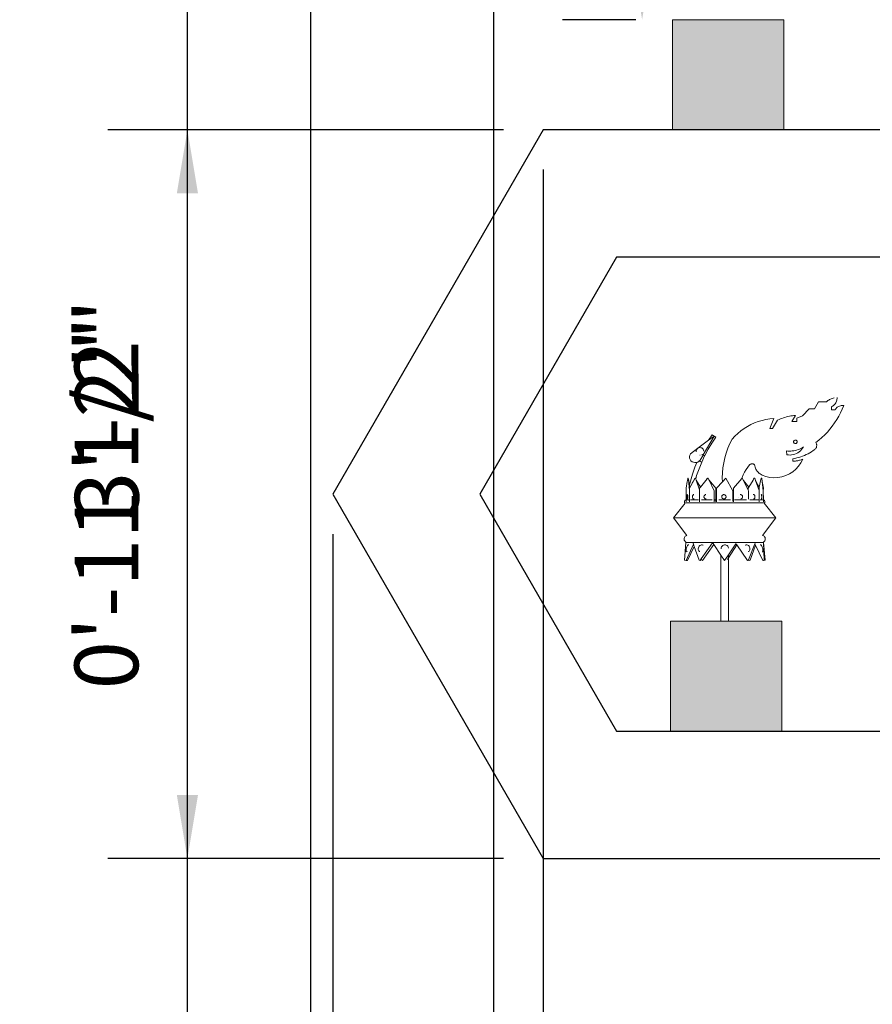
# Model space of a CAD drawing. Units: millimetres. Extents: x 7894 to 8038, y 6851 to 6951.
# Tile 23 of 49: x 7935.52 to 7948.9, y 6916.43 to 6931.89. Entities that reach past the tile are written whole.
import ezdxf

# ---------------------------------------------------------------- set-up
doc = ezdxf.new("R2010")
doc.units = ezdxf.units.MM
for name, color, linetype, lineweight in [('A-ANNO-DIMS', 2, 'Continuous', 18), ('A-FURN-ACCS', 8, 'Continuous', 13), ('A-FURN-CASE', 7, 'Continuous', 30)]:
    doc.layers.add(name, color=color, linetype=linetype, lineweight=lineweight)
doc.layers.add('A-FURN-ACCS-PATT', color=116, linetype='Continuous', lineweight=9, true_color=0x136734)
doc.styles.get("Standard").update_dxf_attribs({"font": 'arial.ttf'})
doc.dimstyles.new('ISO-25', dxfattribs={"dimtxt": 1, "dimasz": 1, "dimexe": 1.25, "dimexo": 0.625, "dimtad": 1, "dimdec": 0, "dimlunit": 4, "dimtxsty": 'Standard', "dimcen": 2.5, "dimclrt": 1, "dimadec": 0, "dimazin": 0, "dimtfac": 1, "dimtdec": 0, "dimtmove": 0, "dimatfit": 3, "dimfxl": 1, "dimarcsym": 0})

# ---------------------------------------------------------------- blocks, each defined once
blk = doc.blocks.new('DISPLAY-LEAF-FINIAL')
for p, q in [((2.209, 3.334), (2.276, 3.441)), ((2.276, 3.441), (2.398, 3.441)), ((2.398, 3.441), (2.409, 3.452)), ((2.409, 3.452), (2.421, 3.461)), ((2.421, 3.461), (2.434, 3.47)), ((2.434, 3.47), (2.447, 3.478)), ((2.447, 3.478), (2.461, 3.485)), ((2.461, 3.485), (2.475, 3.491)), ((2.475, 3.491), (2.489, 3.496)), ((2.489, 3.496), (2.504, 3.501)), ((2.504, 3.501), (2.519, 3.504)), ((2.527, 3.4), (2.516, 3.389)), ((2.536, 3.411), (2.527, 3.4)), ((2.544, 3.424), (2.536, 3.411)), ((2.551, 3.437), (2.544, 3.424)), ((2.556, 3.45), (2.551, 3.437)), ((2.56, 3.465), (2.556, 3.45)), ((2.563, 3.479), (2.56, 3.465)), ((2.565, 3.494), (2.563, 3.479)), ((2.565, 3.508), (2.565, 3.494)), ((2.023, 3.221), (2.127, 3.334)), ((2.127, 3.334), (2.209, 3.334)), ((2.493, 3.371), (2.48, 3.364)), ((2.48, 3.364), (2.48, 3.316)), ((2.48, 3.316), (2.533, 3.316)), ((2.505, 3.379), (2.493, 3.371)), ((2.516, 3.389), (2.505, 3.379)), ((2.533, 3.316), (2.54, 3.327)), ((2.54, 3.327), (2.549, 3.338)), ((2.549, 3.338), (2.558, 3.347)), ((2.558, 3.347), (2.569, 3.356)), ((2.569, 3.356), (2.58, 3.363)), ((2.58, 3.363), (2.592, 3.37)), ((2.62, 3.27), (2.591, 3.216)), ((2.592, 3.37), (2.604, 3.375)), ((2.604, 3.375), (2.617, 3.379)), ((2.617, 3.379), (2.63, 3.382)), ((2.646, 3.325), (2.62, 3.27)), ((2.63, 3.382), (2.643, 3.383)), ((2.643, 3.383), (2.657, 3.383)), ((2.67, 3.382), (2.646, 3.325)), ((2.657, 3.383), (2.67, 3.382)), ((1.213, 3.085), (1.27, 3.111)), ((1.27, 3.111), (1.328, 3.133)), ((1.328, 3.133), (1.388, 3.15)), ((1.388, 3.15), (1.449, 3.164)), ((1.449, 3.164), (1.51, 3.173)), ((1.51, 3.173), (1.572, 3.179)), ((1.572, 3.179), (1.511, 3.024)), ((1.55, 3.024), (1.632, 3.152)), ((1.632, 3.152), (1.654, 3.163)), ((1.654, 3.163), (1.676, 3.173)), ((1.676, 3.173), (1.699, 3.182)), ((1.699, 3.182), (1.722, 3.191)), ((1.722, 3.191), (1.745, 3.198)), ((1.745, 3.198), (1.769, 3.205)), ((1.769, 3.205), (1.793, 3.211)), ((1.793, 3.211), (1.817, 3.216)), ((1.817, 3.216), (1.841, 3.22)), ((1.841, 3.22), (1.865, 3.223)), ((1.914, 3.227), (1.854, 3.133)), ((1.854, 3.133), (1.934, 3.133)), ((1.865, 3.223), (1.889, 3.226)), ((1.889, 3.226), (1.914, 3.227)), ((1.934, 3.185), (2.023, 3.221)), ((1.934, 3.133), (1.934, 3.185)), ((2.527, 3.112), (2.491, 3.062)), ((2.56, 3.163), (2.527, 3.112)), ((2.591, 3.216), (2.56, 3.163)), ((0.962, 2.903), (1.007, 2.946)), ((1.007, 2.946), (1.055, 2.986)), ((1.055, 2.986), (1.105, 3.023)), ((1.105, 3.023), (1.158, 3.056)), ((1.158, 3.056), (1.213, 3.085)), ((1.511, 3.024), (1.55, 3.024)), ((2.413, 2.967), (2.371, 2.923)), ((2.453, 3.014), (2.413, 2.967)), ((2.491, 3.062), (2.453, 3.014)), ((0.547, 2.84), (0.379, 2.713)), ((0.634, 2.9), (0.463, 2.609)), ((0.541, 2.696), (0.599, 2.791)), ((0.605, 2.924), (0.547, 2.84)), ((0.634, 2.905), (0.547, 2.84)), ((0.599, 2.791), (0.663, 2.885)), ((0.634, 2.905), (0.605, 2.924)), ((0.634, 2.9), (0.634, 2.905)), ((0.663, 2.885), (0.634, 2.905)), ((0.884, 2.786), (0.853, 2.713)), ((0.92, 2.857), (0.884, 2.786)), ((0.92, 2.857), (0.962, 2.903)), ((1.883, 2.817), (1.885, 2.824)), ((1.883, 2.81), (1.883, 2.817)), ((1.885, 2.803), (1.883, 2.81)), ((1.885, 2.824), (1.889, 2.831)), ((1.888, 2.797), (1.885, 2.803)), ((1.894, 2.791), (1.888, 2.797)), ((1.889, 2.831), (1.894, 2.836)), ((1.894, 2.836), (1.9, 2.839)), ((1.9, 2.788), (1.894, 2.791)), ((1.9, 2.839), (1.907, 2.841)), ((1.907, 2.786), (1.9, 2.788)), ((1.907, 2.841), (1.914, 2.841)), ((1.914, 2.786), (1.907, 2.786)), ((1.914, 2.841), (1.921, 2.839)), ((1.921, 2.788), (1.914, 2.786)), ((1.921, 2.839), (1.928, 2.836)), ((1.928, 2.791), (1.921, 2.788)), ((1.928, 2.836), (1.933, 2.83)), ((1.933, 2.796), (1.928, 2.791)), ((1.933, 2.83), (1.937, 2.824)), ((1.936, 2.803), (1.933, 2.796)), ((1.938, 2.81), (1.936, 2.803)), ((1.937, 2.824), (1.938, 2.817)), ((1.938, 2.817), (1.938, 2.81)), ((2.281, 2.839), (2.233, 2.801)), ((2.233, 2.801), (2.238, 2.792)), ((2.238, 2.792), (2.242, 2.783)), ((2.242, 2.783), (2.245, 2.774)), ((2.327, 2.88), (2.281, 2.839)), ((2.371, 2.923), (2.327, 2.88)), ((0.264, 2.627), (0.253, 2.607)), ((0.379, 2.713), (0.264, 2.627)), ((0.353, 2.675), (0.358, 2.69)), ((0.353, 2.66), (0.353, 2.675)), ((0.353, 2.659), (0.353, 2.66)), ((0.353, 2.657), (0.353, 2.659)), ((0.358, 2.69), (0.367, 2.703)), ((0.367, 2.703), (0.379, 2.713)), ((0.379, 2.713), (0.393, 2.72)), ((0.393, 2.72), (0.409, 2.723)), ((0.409, 2.723), (0.425, 2.722)), ((0.425, 2.722), (0.44, 2.718)), ((0.44, 2.718), (0.453, 2.709)), ((0.453, 2.709), (0.464, 2.698)), ((0.464, 2.698), (0.471, 2.684)), ((0.471, 2.684), (0.475, 2.669)), ((0.474, 2.667), (0.475, 2.669)), ((0.474, 2.667), (0.475, 2.666)), ((0.541, 2.696), (0.488, 2.597)), ((0.826, 2.638), (0.804, 2.562)), ((0.853, 2.713), (0.826, 2.638)), ((1.793, 2.668), (1.77, 2.67)), ((1.77, 2.67), (1.776, 2.611)), ((1.816, 2.667), (1.793, 2.668)), ((1.84, 2.668), (1.816, 2.667)), ((1.863, 2.67), (1.84, 2.668)), ((1.886, 2.673), (1.863, 2.67)), ((1.909, 2.678), (1.886, 2.673)), ((1.926, 2.63), (1.902, 2.62)), ((1.931, 2.684), (1.909, 2.678)), ((1.949, 2.642), (1.926, 2.63)), ((1.954, 2.692), (1.931, 2.684)), ((1.97, 2.657), (1.949, 2.642)), ((1.975, 2.701), (1.954, 2.692)), ((1.99, 2.673), (1.97, 2.657)), ((1.996, 2.711), (1.975, 2.701)), ((2.007, 2.692), (1.99, 2.673)), ((2.017, 2.722), (1.996, 2.711)), ((2.023, 2.712), (2.007, 2.692)), ((2.036, 2.734), (2.017, 2.722)), ((2.036, 2.734), (2.023, 2.712)), ((2.11, 2.627), (2.082, 2.613)), ((2.137, 2.643), (2.11, 2.627)), ((2.164, 2.659), (2.137, 2.643)), ((2.19, 2.677), (2.164, 2.659)), ((2.216, 2.695), (2.19, 2.677)), ((2.223, 2.702), (2.216, 2.695)), ((2.23, 2.709), (2.223, 2.702)), ((2.235, 2.717), (2.23, 2.709)), ((2.24, 2.726), (2.235, 2.717)), ((2.243, 2.735), (2.24, 2.726)), ((2.245, 2.745), (2.243, 2.735)), ((2.245, 2.774), (2.246, 2.764)), ((2.246, 2.754), (2.245, 2.745)), ((2.246, 2.764), (2.246, 2.754)), ((0.253, 2.607), (0.249, 2.584)), ((0.249, 2.58), (0.249, 2.584)), ((0.249, 2.58), (0.251, 2.557)), ((0.251, 2.557), (0.259, 2.536)), ((0.259, 2.536), (0.272, 2.517)), ((0.272, 2.517), (0.29, 2.502)), ((0.29, 2.502), (0.311, 2.492)), ((0.311, 2.492), (0.334, 2.488)), ((0.363, 2.491), (0.332, 2.415)), ((0.334, 2.488), (0.358, 2.489)), ((0.358, 2.489), (0.363, 2.491)), ((0.363, 2.491), (0.38, 2.497)), ((0.365, 2.496), (0.363, 2.491)), ((0.38, 2.497), (0.4, 2.51)), ((0.398, 2.513), (0.402, 2.512)), ((0.398, 2.391), (0.44, 2.495)), ((0.403, 2.513), (0.4, 2.514)), ((0.4, 2.51), (0.402, 2.512)), ((0.402, 2.512), (0.403, 2.513)), ((0.402, 2.512), (0.44, 2.495)), ((0.403, 2.513), (0.415, 2.527)), ((0.403, 2.513), (0.44, 2.496)), ((0.409, 2.511), (0.408, 2.509)), ((0.42, 2.535), (0.409, 2.511)), ((0.414, 2.606), (0.413, 2.603)), ((0.461, 2.605), (0.415, 2.527)), ((0.44, 2.496), (0.486, 2.593)), ((0.443, 2.613), (0.446, 2.612)), ((0.451, 2.615), (0.449, 2.616)), ((0.463, 2.609), (0.461, 2.605)), ((0.486, 2.593), (0.461, 2.605)), ((0.463, 2.609), (0.488, 2.597)), ((0.787, 2.485), (0.774, 2.406)), ((0.804, 2.562), (0.787, 2.485)), ((1.801, 2.608), (1.776, 2.611)), ((1.827, 2.607), (1.801, 2.608)), ((1.852, 2.609), (1.827, 2.607)), ((1.878, 2.613), (1.852, 2.609)), ((1.903, 2.554), (1.872, 2.548)), ((1.872, 2.548), (1.872, 2.508)), ((1.872, 2.508), (1.885, 2.509)), ((1.902, 2.62), (1.878, 2.613)), ((1.885, 2.509), (1.898, 2.51)), ((1.898, 2.51), (1.911, 2.511)), ((1.934, 2.561), (1.903, 2.554)), ((1.911, 2.511), (1.924, 2.513)), ((1.924, 2.513), (1.937, 2.515)), ((1.964, 2.569), (1.934, 2.561)), ((1.937, 2.515), (1.95, 2.518)), ((1.95, 2.518), (1.963, 2.521)), ((1.997, 2.484), (1.961, 2.432)), ((1.963, 2.521), (1.976, 2.524)), ((1.994, 2.578), (1.964, 2.569)), ((1.976, 2.524), (1.988, 2.528)), ((1.988, 2.528), (2.001, 2.532)), ((2.024, 2.588), (1.994, 2.578)), ((2.026, 2.541), (1.997, 2.484)), ((2.001, 2.532), (2.013, 2.536)), ((2.013, 2.536), (2.026, 2.541)), ((2.053, 2.6), (2.024, 2.588)), ((2.082, 2.613), (2.053, 2.6)), ((0.332, 2.415), (0.295, 2.306)), ((0.361, 2.285), (0.398, 2.391)), ((0.766, 2.327), (0.763, 2.248)), ((0.774, 2.406), (0.766, 2.327)), ((1.113, 2.339), (1.092, 2.297)), ((1.136, 2.379), (1.113, 2.339)), ((1.163, 2.417), (1.136, 2.379)), ((1.193, 2.452), (1.163, 2.417)), ((1.198, 2.457), (1.193, 2.452)), ((1.204, 2.462), (1.198, 2.457)), ((1.211, 2.465), (1.204, 2.462)), ((1.218, 2.467), (1.211, 2.465)), ((1.225, 2.469), (1.218, 2.467)), ((1.232, 2.47), (1.225, 2.469)), ((1.239, 2.469), (1.232, 2.47)), ((1.247, 2.467), (1.239, 2.469)), ((1.254, 2.465), (1.247, 2.467)), ((1.26, 2.462), (1.254, 2.465)), ((1.266, 2.457), (1.26, 2.462)), ((1.271, 2.452), (1.266, 2.457)), ((1.274, 2.435), (1.271, 2.452)), ((1.278, 2.418), (1.274, 2.435)), ((1.283, 2.402), (1.278, 2.418)), ((1.29, 2.386), (1.283, 2.402)), ((1.298, 2.371), (1.29, 2.386)), ((1.308, 2.357), (1.298, 2.371)), ((1.319, 2.343), (1.308, 2.357)), ((1.331, 2.331), (1.319, 2.343)), ((1.343, 2.319), (1.331, 2.331)), ((1.357, 2.309), (1.343, 2.319)), ((1.87, 2.344), (1.816, 2.31)), ((1.918, 2.385), (1.87, 2.344)), ((1.961, 2.432), (1.918, 2.385)), ((0.213, 2.19), (0.195, 2.086)), ((0.213, 2.19), (0.215, 2.201)), ((0.215, 2.201), (0.22, 2.245)), ((0.223, 2.245), (0.215, 2.201)), ((0.223, 2.245), (0.22, 2.245)), ((0.223, 2.245), (0.23, 2.245)), ((0.232, 2.22), (0.23, 2.245)), ((0.232, 2.22), (0.25, 2.138)), ((0.244, 2.11), (0.232, 2.22)), ((0.317, 2.207), (0.248, 2.086)), ((0.263, 2.194), (0.25, 2.138)), ((0.295, 2.306), (0.263, 2.194)), ((0.297, 2.185), (0.292, 2.162)), ((0.317, 2.207), (0.33, 2.245)), ((0.338, 2.245), (0.317, 2.207)), ((0.332, 2.245), (0.33, 2.245)), ((0.344, 2.245), (0.338, 2.245)), ((0.347, 2.235), (0.344, 2.245)), ((0.347, 2.235), (0.361, 2.285)), ((0.354, 2.213), (0.347, 2.235)), ((0.354, 2.213), (0.42, 2.104)), ((0.404, 2.061), (0.354, 2.213)), ((0.507, 2.209), (0.42, 2.104)), ((0.507, 2.209), (0.525, 2.245)), ((0.532, 2.239), (0.507, 2.209)), ((0.528, 2.245), (0.525, 2.245)), ((0.528, 2.245), (0.532, 2.239)), ((0.537, 2.245), (0.532, 2.239)), ((0.54, 2.245), (0.537, 2.245)), ((0.556, 2.211), (0.54, 2.245)), ((0.548, 2.22), (0.556, 2.211)), ((0.556, 2.211), (0.663, 2.086)), ((0.636, 2.045), (0.556, 2.211)), ((0.765, 2.186), (0.671, 2.086)), ((0.763, 2.248), (0.765, 2.186)), ((0.821, 2.245), (0.765, 2.186)), ((0.93, 2.045), (0.821, 2.245)), ((1.07, 2.239), (0.939, 2.086)), ((1.07, 2.239), (1.069, 2.235)), ((1.071, 2.24), (1.07, 2.239)), ((1.07, 2.239), (1.071, 2.237)), ((1.075, 2.254), (1.071, 2.24)), ((1.074, 2.245), (1.071, 2.24)), ((1.074, 2.245), (1.078, 2.245)), ((1.092, 2.297), (1.075, 2.254)), ((1.095, 2.209), (1.078, 2.245)), ((1.095, 2.209), (1.182, 2.104)), ((1.095, 2.209), (1.171, 2.054)), ((1.248, 2.213), (1.182, 2.104)), ((1.248, 2.213), (1.258, 2.245)), ((1.265, 2.242), (1.248, 2.213)), ((1.258, 2.245), (1.264, 2.245)), ((1.264, 2.245), (1.265, 2.242)), ((1.267, 2.245), (1.265, 2.242)), ((1.267, 2.245), (1.272, 2.245)), ((1.285, 2.207), (1.272, 2.245)), ((1.285, 2.207), (1.344, 2.103)), ((1.285, 2.207), (1.34, 2.048)), ((1.37, 2.22), (1.344, 2.103)), ((1.372, 2.3), (1.357, 2.309)), ((1.37, 2.22), (1.372, 2.245)), ((1.375, 2.245), (1.37, 2.22)), ((1.387, 2.292), (1.372, 2.3)), ((1.372, 2.245), (1.375, 2.245)), ((1.375, 2.245), (1.382, 2.245)), ((1.382, 2.245), (1.389, 2.19)), ((1.447, 2.27), (1.387, 2.292)), ((1.389, 2.19), (1.408, 2.086)), ((1.407, 2.045), (1.389, 2.19)), ((1.509, 2.256), (1.447, 2.27)), ((1.572, 2.25), (1.509, 2.256)), ((1.635, 2.253), (1.572, 2.25)), ((1.698, 2.264), (1.635, 2.253)), ((1.759, 2.283), (1.698, 2.264)), ((1.816, 2.31), (1.759, 2.283)), ((0.195, 2.086), (0.195, 2.048)), ((0.195, 2.045), (0.195, 2.048)), ((0.195, 2.045), (0.195, 1.903)), ((0.244, 2.11), (0.239, 2.089)), ((0.25, 2.138), (0.244, 2.11)), ((0.248, 2.065), (0.244, 2.11)), ((0.248, 2.086), (0.248, 2.065)), ((0.248, 2.065), (0.248, 1.903)), ((0.25, 2.138), (0.256, 2.115)), ((0.42, 2.104), (0.404, 2.086)), ((0.404, 2.086), (0.404, 2.061)), ((0.404, 2.061), (0.404, 1.901)), ((0.636, 2.045), (0.637, 1.903)), ((0.663, 2.086), (0.663, 1.903)), ((0.671, 2.086), (0.671, 1.903)), ((0.93, 2.045), (0.931, 1.934)), ((0.939, 2.086), (0.939, 1.934)), ((1.182, 2.104), (1.171, 2.086)), ((1.171, 2.086), (1.171, 2.054)), ((1.176, 2.045), (1.171, 2.054)), ((1.176, 2.045), (1.177, 1.914)), ((1.344, 2.103), (1.34, 2.086)), ((1.34, 2.086), (1.34, 2.048)), ((1.341, 2.045), (1.34, 2.048)), ((1.341, 2.045), (1.342, 1.903)), ((1.408, 2.086), (1.407, 2.045)), ((1.407, 2.045), (1.408, 1.903)), ((0.17, 1.877), (0.172, 1.885)), ((0.17, 1.87), (0.17, 1.877)), ((0.172, 1.862), (0.17, 1.87)), ((0.172, 1.885), (0.176, 1.892)), ((0.175, 1.855), (0.172, 1.862)), ((0.181, 1.849), (0.175, 1.855)), ((0.176, 1.892), (0.182, 1.898)), ((0.182, 1.898), (0.189, 1.901)), ((0.189, 1.901), (0.195, 1.903)), ((0.195, 1.903), (0.195, 1.901)), ((0.195, 1.903), (0.196, 1.903)), ((0.195, 1.898), (0.195, 1.87)), ((0.195, 1.862), (0.195, 1.855)), ((0.195, 1.855), (0.195, 1.855)), ((0.205, 1.855), (0.195, 1.855)), ((0.196, 1.903), (0.198, 1.903)), ((0.196, 1.903), (0.197, 1.903)), ((0.237, 1.903), (0.198, 1.903)), ((0.205, 1.855), (0.205, 1.851)), ((0.248, 1.855), (0.205, 1.855)), ((0.207, 1.965), (0.208, 1.973)), ((0.207, 1.956), (0.207, 1.965)), ((0.207, 1.947), (0.207, 1.956)), ((0.207, 1.938), (0.207, 1.947)), ((0.208, 1.93), (0.207, 1.938)), ((0.208, 1.973), (0.209, 1.979)), ((0.209, 1.924), (0.208, 1.93)), ((0.209, 1.979), (0.211, 1.984)), ((0.211, 1.919), (0.209, 1.924)), ((0.21, 1.956), (0.211, 1.965)), ((0.21, 1.947), (0.21, 1.956)), ((0.211, 1.938), (0.21, 1.947)), ((0.211, 1.984), (0.213, 1.986)), ((0.211, 1.965), (0.212, 1.973)), ((0.212, 1.93), (0.211, 1.938)), ((0.213, 1.917), (0.211, 1.919)), ((0.212, 1.973), (0.213, 1.979)), ((0.213, 1.924), (0.212, 1.93)), ((0.216, 1.986), (0.213, 1.986)), ((0.213, 1.979), (0.214, 1.984)), ((0.216, 1.947), (0.213, 1.924)), ((0.214, 1.919), (0.213, 1.924)), ((0.214, 1.917), (0.213, 1.917)), ((0.214, 1.984), (0.216, 1.986)), ((0.216, 1.917), (0.214, 1.919)), ((0.216, 1.917), (0.214, 1.917)), ((0.217, 1.965), (0.216, 1.956)), ((0.216, 1.956), (0.216, 1.947)), ((0.216, 1.947), (0.217, 1.938)), ((0.218, 1.917), (0.216, 1.917)), ((0.218, 1.973), (0.217, 1.965)), ((0.218, 1.967), (0.217, 1.965)), ((0.217, 1.938), (0.218, 1.93)), ((0.219, 1.979), (0.218, 1.973)), ((0.218, 1.973), (0.218, 1.967)), ((0.218, 1.93), (0.219, 1.924)), ((0.22, 1.981), (0.219, 1.979)), ((0.22, 1.981), (0.219, 1.979)), ((0.219, 1.924), (0.22, 1.921)), ((0.221, 1.973), (0.22, 1.965)), ((0.22, 1.965), (0.22, 1.956)), ((0.22, 1.956), (0.22, 1.947)), ((0.22, 1.947), (0.22, 1.938)), ((0.22, 1.938), (0.221, 1.93)), ((0.222, 1.975), (0.221, 1.973)), ((0.221, 1.93), (0.222, 1.928)), ((0.24, 1.855), (0.24, 1.849)), ((0.248, 1.903), (0.244, 1.903)), ((0.245, 1.898), (0.244, 1.886)), ((0.248, 1.897), (0.244, 1.897)), ((0.248, 1.925), (0.246, 1.901)), ((0.248, 1.903), (0.248, 1.901)), ((0.248, 1.898), (0.248, 1.897)), ((0.248, 1.897), (0.248, 1.87)), ((0.248, 1.862), (0.248, 1.855)), ((0.248, 1.855), (0.276, 1.855)), ((0.391, 1.903), (0.265, 1.903)), ((0.275, 1.849), (0.276, 1.855)), ((0.276, 1.855), (0.405, 1.855)), ((0.295, 1.956), (0.297, 1.965)), ((0.295, 1.947), (0.295, 1.956)), ((0.297, 1.938), (0.295, 1.947)), ((0.297, 1.965), (0.3, 1.973)), ((0.3, 1.93), (0.297, 1.938)), ((0.3, 1.973), (0.304, 1.979)), ((0.303, 1.924), (0.3, 1.93)), ((0.308, 1.919), (0.303, 1.924)), ((0.304, 1.979), (0.308, 1.984)), ((0.308, 1.984), (0.314, 1.986)), ((0.313, 1.917), (0.308, 1.919)), ((0.319, 1.917), (0.313, 1.917)), ((0.316, 1.986), (0.314, 1.986)), ((0.322, 1.917), (0.319, 1.917)), ((0.404, 1.898), (0.404, 1.87)), ((0.404, 1.862), (0.405, 1.855)), ((0.405, 1.855), (0.637, 1.855)), ((0.439, 1.903), (0.607, 1.903)), ((0.476, 1.956), (0.478, 1.965)), ((0.476, 1.947), (0.476, 1.956)), ((0.478, 1.938), (0.476, 1.947)), ((0.478, 1.965), (0.482, 1.973)), ((0.482, 1.93), (0.478, 1.938)), ((0.482, 1.973), (0.488, 1.979)), ((0.488, 1.924), (0.482, 1.93)), ((0.488, 1.979), (0.495, 1.984)), ((0.495, 1.919), (0.488, 1.924)), ((0.495, 1.984), (0.502, 1.986)), ((0.502, 1.917), (0.495, 1.919)), ((0.504, 1.986), (0.502, 1.986)), ((0.51, 1.917), (0.502, 1.917)), ((0.512, 1.917), (0.51, 1.917)), ((0.637, 1.903), (0.634, 1.903)), ((0.637, 1.897), (0.634, 1.897)), ((0.637, 1.903), (0.637, 1.901)), ((0.663, 1.903), (0.637, 1.903)), ((0.637, 1.898), (0.637, 1.897)), ((0.637, 1.897), (0.637, 1.87)), ((0.663, 1.897), (0.637, 1.897)), ((0.637, 1.862), (0.637, 1.855)), ((0.663, 1.855), (0.637, 1.855)), ((0.663, 1.903), (0.671, 1.903)), ((0.663, 1.903), (0.663, 1.901)), ((0.663, 1.898), (0.663, 1.897)), ((0.663, 1.897), (0.663, 1.87)), ((0.671, 1.897), (0.663, 1.897)), ((0.663, 1.862), (0.663, 1.855)), ((0.671, 1.903), (0.671, 1.901)), ((0.671, 1.898), (0.671, 1.897)), ((0.671, 1.897), (0.671, 1.87)), ((0.671, 1.862), (0.671, 1.855)), ((0.671, 1.855), (0.932, 1.855)), ((0.708, 1.903), (0.894, 1.903)), ((0.754, 1.956), (0.756, 1.965)), ((0.754, 1.947), (0.754, 1.956)), ((0.756, 1.938), (0.754, 1.947)), ((0.756, 1.965), (0.761, 1.973)), ((0.761, 1.93), (0.756, 1.938)), ((0.761, 1.973), (0.767, 1.979)), ((0.767, 1.924), (0.761, 1.93)), ((0.767, 1.979), (0.775, 1.984)), ((0.775, 1.919), (0.767, 1.924)), ((0.775, 1.984), (0.784, 1.986)), ((0.784, 1.917), (0.775, 1.919)), ((0.784, 1.986), (0.793, 1.986)), ((0.793, 1.917), (0.784, 1.917)), ((0.793, 1.986), (0.802, 1.984)), ((0.802, 1.919), (0.793, 1.917)), ((0.802, 1.984), (0.81, 1.979)), ((0.81, 1.924), (0.802, 1.919)), ((0.81, 1.979), (0.816, 1.973)), ((0.816, 1.93), (0.81, 1.924)), ((0.816, 1.973), (0.821, 1.965)), ((0.821, 1.938), (0.816, 1.93)), ((0.821, 1.965), (0.823, 1.956)), ((0.823, 1.947), (0.821, 1.938)), ((0.823, 1.956), (0.823, 1.947)), ((0.939, 1.934), (0.931, 1.934)), ((0.931, 1.934), (0.931, 1.903)), ((0.931, 1.903), (0.931, 1.901)), ((0.939, 1.903), (0.931, 1.903)), ((0.931, 1.898), (0.931, 1.897)), ((0.931, 1.897), (0.932, 1.87)), ((0.939, 1.897), (0.931, 1.897)), ((0.932, 1.862), (0.932, 1.855)), ((0.939, 1.855), (0.932, 1.855)), ((0.942, 1.934), (0.939, 1.934)), ((0.939, 1.934), (0.939, 1.903)), ((0.942, 1.903), (0.939, 1.903)), ((0.939, 1.903), (0.939, 1.901)), ((0.939, 1.898), (0.939, 1.897)), ((0.942, 1.897), (0.939, 1.897)), ((0.939, 1.897), (0.939, 1.87)), ((0.939, 1.862), (0.939, 1.855)), ((1.342, 1.855), (0.939, 1.855)), ((0.953, 1.903), (1.146, 1.903)), ((1.022, 1.935), (1.021, 1.935)), ((1.044, 1.986), (1.046, 1.986)), ((1.046, 1.986), (1.054, 1.986)), ((1.052, 1.917), (1.054, 1.917)), ((1.054, 1.986), (1.062, 1.984)), ((1.062, 1.919), (1.054, 1.917)), ((1.062, 1.984), (1.069, 1.979)), ((1.069, 1.924), (1.062, 1.919)), ((1.069, 1.979), (1.075, 1.973)), ((1.075, 1.93), (1.069, 1.924)), ((1.075, 1.973), (1.079, 1.965)), ((1.079, 1.938), (1.075, 1.93)), ((1.079, 1.965), (1.081, 1.956)), ((1.081, 1.947), (1.079, 1.938)), ((1.081, 1.956), (1.081, 1.947)), ((1.33, 1.903), (1.197, 1.903)), ((1.249, 1.986), (1.251, 1.986)), ((1.251, 1.986), (1.257, 1.986)), ((1.254, 1.917), (1.257, 1.917)), ((1.257, 1.986), (1.263, 1.984)), ((1.263, 1.919), (1.257, 1.917)), ((1.263, 1.984), (1.268, 1.979)), ((1.268, 1.924), (1.263, 1.919)), ((1.268, 1.979), (1.272, 1.973)), ((1.272, 1.93), (1.268, 1.924)), ((1.272, 1.973), (1.275, 1.965)), ((1.275, 1.938), (1.272, 1.93)), ((1.275, 1.965), (1.276, 1.956)), ((1.276, 1.947), (1.275, 1.938)), ((1.276, 1.956), (1.276, 1.947)), ((1.347, 1.903), (1.342, 1.903)), ((1.342, 1.903), (1.342, 1.901)), ((1.342, 1.898), (1.342, 1.897)), ((1.347, 1.897), (1.342, 1.897)), ((1.342, 1.897), (1.342, 1.87)), ((1.342, 1.862), (1.342, 1.855)), ((1.408, 1.855), (1.342, 1.855)), ((1.356, 1.903), (1.4, 1.903)), ((1.373, 1.986), (1.376, 1.986)), ((1.378, 1.919), (1.375, 1.917)), ((1.375, 1.917), (1.379, 1.917)), ((1.376, 1.986), (1.378, 1.984)), ((1.376, 1.986), (1.377, 1.986)), ((1.377, 1.986), (1.379, 1.986)), ((1.378, 1.984), (1.379, 1.979)), ((1.379, 1.924), (1.378, 1.919)), ((1.379, 1.986), (1.381, 1.984)), ((1.379, 1.979), (1.381, 1.973)), ((1.381, 1.93), (1.379, 1.924)), ((1.381, 1.919), (1.379, 1.917)), ((1.381, 1.984), (1.383, 1.979)), ((1.381, 1.973), (1.382, 1.965)), ((1.382, 1.938), (1.381, 1.93)), ((1.383, 1.924), (1.381, 1.919)), ((1.382, 1.965), (1.382, 1.956)), ((1.382, 1.956), (1.382, 1.947)), ((1.382, 1.947), (1.382, 1.938)), ((1.383, 1.979), (1.384, 1.973)), ((1.384, 1.93), (1.383, 1.924)), ((1.384, 1.973), (1.385, 1.965)), ((1.385, 1.938), (1.384, 1.93)), ((1.385, 1.965), (1.386, 1.956)), ((1.386, 1.947), (1.385, 1.938)), ((1.386, 1.956), (1.386, 1.947)), ((1.408, 1.903), (1.413, 1.901)), ((1.408, 1.903), (1.408, 1.901)), ((1.408, 1.898), (1.408, 1.87)), ((1.408, 1.862), (1.408, 1.855)), ((1.413, 1.901), (1.42, 1.898)), ((1.42, 1.898), (1.426, 1.892)), ((1.427, 1.855), (1.421, 1.849)), ((1.426, 1.892), (1.43, 1.885)), ((1.431, 1.862), (1.427, 1.855)), ((1.43, 1.885), (1.432, 1.877)), ((1.433, 1.87), (1.431, 1.862)), ((1.432, 1.877), (1.433, 1.87)), ((0, 1.62), (0.181, 1.849)), ((0.205, 1.851), (0.205, 1.849)), ((1.421, 1.849), (1.602, 1.62)), ((0.207, 1.343), (0, 1.62)), ((1.602, 1.62), (0, 1.62)), ((1.602, 1.62), (1.395, 1.343)), ((0.164, 1.297), (0.168, 1.31)), ((0.164, 1.283), (0.164, 1.297)), ((0.167, 1.27), (0.164, 1.283)), ((0.173, 1.258), (0.167, 1.27)), ((0.168, 1.31), (0.174, 1.321)), ((0.182, 1.248), (0.173, 1.258)), ((0.174, 1.321), (0.183, 1.331)), ((0.193, 1.24), (0.182, 1.248)), ((0.183, 1.331), (0.195, 1.338)), ((0.206, 1.236), (0.193, 1.24)), ((0.195, 1.338), (0.207, 1.343)), ((1.395, 1.343), (1.408, 1.338)), ((1.409, 1.24), (1.397, 1.236)), ((1.408, 1.338), (1.419, 1.331)), ((1.42, 1.248), (1.409, 1.24)), ((1.419, 1.331), (1.428, 1.321)), ((1.429, 1.258), (1.42, 1.248)), ((1.428, 1.321), (1.434, 1.31)), ((1.435, 1.27), (1.429, 1.258)), ((1.434, 1.31), (1.438, 1.297)), ((1.438, 1.283), (1.435, 1.27)), ((1.438, 1.297), (1.438, 1.283)), ((0.171, 0.955), (0.191, 1.234)), ((0.219, 1.234), (0.191, 1.234)), ((0.194, 1.111), (0.196, 1.124)), ((0.195, 1.101), (0.194, 1.111)), ((0.196, 1.094), (0.195, 1.101)), ((0.196, 0.954), (0.311, 1.21)), ((0.196, 1.124), (0.198, 1.137)), ((0.199, 1.09), (0.196, 1.094)), ((0.198, 1.137), (0.202, 1.152)), ((0.203, 1.089), (0.199, 1.09)), ((0.202, 1.152), (0.206, 1.165)), ((0.204, 1.088), (0.203, 1.089)), ((0.219, 1.234), (0.206, 1.236)), ((0.206, 1.165), (0.212, 1.177)), ((0.211, 1.096), (0.213, 1.092)), ((0.212, 1.177), (0.217, 1.187)), ((0.213, 1.092), (0.214, 1.092)), ((0.214, 1.1), (0.214, 1.098)), ((0.215, 0.949), (0.324, 1.172)), ((0.217, 1.187), (0.223, 1.193)), ((0.219, 1.234), (0.297, 1.234)), ((0.223, 1.193), (0.228, 1.197)), ((0.228, 1.197), (0.232, 1.196)), ((0.232, 1.195), (0.232, 1.196)), ((0.232, 1.195), (0.237, 1.195)), ((0.297, 1.234), (0.302, 1.234)), ((0.303, 1.232), (0.297, 1.234)), ((0.303, 1.232), (0.302, 1.234)), ((0.302, 1.234), (0.594, 1.234)), ((0.311, 1.21), (0.303, 1.232)), ((0.324, 1.172), (0.311, 1.21)), ((0.402, 0.955), (0.324, 1.172)), ((0.387, 1.137), (0.389, 1.152)), ((0.387, 1.124), (0.387, 1.137)), ((0.391, 1.111), (0.387, 1.124)), ((0.389, 1.152), (0.395, 1.165)), ((0.397, 1.101), (0.391, 1.111)), ((0.395, 1.165), (0.403, 1.177)), ((0.406, 1.094), (0.397, 1.101)), ((0.403, 1.177), (0.413, 1.187)), ((0.409, 1.092), (0.406, 1.094)), ((0.413, 1.187), (0.424, 1.193)), ((0.424, 1.193), (0.436, 1.197)), ((0.434, 0.975), (0.609, 1.228)), ((0.436, 1.197), (0.448, 1.196)), ((0.448, 1.196), (0.458, 1.192)), ((0.455, 0.949), (0.632, 1.205)), ((0.458, 1.192), (0.461, 1.191)), ((0.594, 1.234), (0.617, 1.234)), ((0.609, 1.228), (0.594, 1.234)), ((0.617, 1.228), (0.617, 1.234)), ((0.952, 1.234), (0.617, 1.234)), ((0.632, 1.205), (0.617, 1.228)), ((0.742, 1.037), (0.632, 1.205)), ((0.747, 1.137), (0.748, 1.152)), ((0.747, 1.136), (0.747, 1.137)), ((0.748, 1.152), (0.752, 1.165)), ((0.752, 1.165), (0.76, 1.177)), ((0.76, 1.177), (0.77, 1.187)), ((0.77, 1.187), (0.783, 1.193)), ((0.783, 1.193), (0.797, 1.197)), ((0.797, 1.197), (0.812, 1.196)), ((0.812, 1.196), (0.826, 1.192)), ((0.826, 1.192), (0.838, 1.185)), ((0.838, 1.185), (0.848, 1.175)), ((0.848, 1.175), (0.855, 1.162)), ((0.855, 1.162), (0.859, 1.148)), ((0.859, 1.147), (0.859, 1.148)), ((0.86, 1.041), (0.977, 1.215)), ((0.86, 0.992), (0.99, 1.195)), ((0.981, 1.234), (0.952, 1.234)), ((0.977, 1.215), (0.974, 1.218)), ((0.99, 1.195), (0.977, 1.215)), ((0.981, 1.234), (0.982, 1.234)), ((0.982, 1.234), (0.983, 1.234)), ((1.284, 1.234), (0.983, 1.234)), ((1.16, 0.949), (0.99, 1.195)), ((1.124, 1.192), (1.126, 1.193)), ((1.126, 1.193), (1.127, 1.193)), ((1.127, 1.193), (1.138, 1.197)), ((1.138, 1.197), (1.15, 1.196)), ((1.15, 1.196), (1.162, 1.192)), ((1.162, 1.192), (1.174, 1.185)), ((1.174, 1.092), (1.172, 1.091)), ((1.174, 1.185), (1.184, 1.175)), ((1.174, 1.092), (1.175, 1.092)), ((1.185, 1.099), (1.175, 1.092)), ((1.177, 0.964), (1.275, 1.212)), ((1.184, 1.175), (1.191, 1.162)), ((1.192, 1.109), (1.185, 1.099)), ((1.191, 1.162), (1.196, 1.148)), ((1.196, 1.121), (1.192, 1.109)), ((1.196, 1.148), (1.198, 1.134)), ((1.198, 1.134), (1.196, 1.121)), ((1.202, 0.955), (1.285, 1.19)), ((1.275, 1.212), (1.283, 1.232)), ((1.285, 1.19), (1.275, 1.212)), ((1.283, 1.232), (1.29, 1.234)), ((1.283, 1.232), (1.284, 1.234)), ((1.284, 1.234), (1.29, 1.234)), ((1.398, 0.949), (1.285, 1.19)), ((1.29, 1.234), (1.383, 1.234)), ((1.359, 1.195), (1.364, 1.197)), ((1.359, 1.195), (1.362, 1.195)), ((1.364, 1.197), (1.369, 1.196)), ((1.369, 1.196), (1.374, 1.192)), ((1.374, 1.192), (1.38, 1.185)), ((1.38, 1.185), (1.386, 1.175)), ((1.397, 1.236), (1.383, 1.234)), ((1.41, 1.234), (1.383, 1.234)), ((1.386, 1.175), (1.392, 1.162)), ((1.392, 1.089), (1.39, 1.088)), ((1.39, 1.088), (1.395, 1.089)), ((1.392, 1.162), (1.396, 1.148)), ((1.399, 1.092), (1.395, 1.089)), ((1.396, 1.148), (1.4, 1.134)), ((1.401, 1.099), (1.399, 1.092)), ((1.4, 1.134), (1.402, 1.121)), ((1.402, 1.109), (1.401, 1.099)), ((1.402, 1.121), (1.402, 1.109)), ((1.411, 1.234), (1.41, 1.234)), ((1.411, 1.232), (1.411, 1.234)), ((1.435, 0.955), (1.411, 1.232)), ((1.42, 0.955), (1.411, 1.232)), ((0.194, 0.949), (0.171, 0.955)), ((0.194, 0.949), (0.196, 0.954)), ((0.215, 0.949), (0.196, 0.954)), ((0.416, 0.949), (0.402, 0.955)), ((0.416, 0.949), (0.434, 0.975)), ((0.442, 0.955), (0.434, 0.975)), ((0.455, 0.949), (0.442, 0.955)), ((0.742, 0), (0.742, 1.037)), ((0.799, 0.949), (0.742, 1.037)), ((0.799, 0.949), (0.816, 0.974)), ((0.816, 0.974), (0.814, 0.977)), ((0.816, 0.974), (0.86, 1.041)), ((0.816, 0.973), (0.816, 0.974)), ((0.843, 0.965), (0.86, 0.992)), ((0.86, 1.041), (0.86, 1.047)), ((0.86, 0.992), (0.86, 1.041)), ((0.86, 0), (0.86, 0.992)), ((1.16, 0.949), (1.173, 0.955)), ((1.173, 0.955), (1.177, 0.964)), ((1.187, 0.949), (1.177, 0.964)), ((1.187, 0.949), (1.202, 0.955)), ((1.398, 0.949), (1.41, 0.953)), ((1.41, 0.953), (1.42, 0.955)), ((1.412, 0.949), (1.41, 0.953)), ((1.412, 0.949), (1.435, 0.955))]:
    blk.add_line(p, q)
blk = doc.blocks.new('*D17')
at = {"layer": 'A-ANNO-DIMS', "color": 0, "lineweight": -2, "transparency": 16777216}
for p, q in [((7945.291, 6935.394), (7945.291, 6950.748)), ((7945.192, 6935.394), (7944.041, 6935.394)), ((7945.291, 6932.885), (7945.291, 6934.394)), ((7945.192, 6931.885), (7944.041, 6931.885))]:
    blk.add_line(p, q, dxfattribs=at)
at = {"layer": 'A-ANNO-DIMS', "color": 0, "transparency": 16777216}
for points in [[(7945.124, 6934.394), (7945.457, 6934.394), (7945.291, 6935.394)], [(7945.124, 6932.885), (7945.457, 6932.885), (7945.291, 6931.885)]]:
    blk.add_solid(points, dxfattribs=at)
at = {"layer": 'Defpoints', "color": 0, "transparency": 16777216}
for p in [(7945.291, 6935.394), (7945.817, 6935.394), (7945.817, 6931.885)]:
    blk.add_point(p, dxfattribs=at)
at = {"layer": 'A-ANNO-DIMS', "color": 1, "transparency": 16777216, "insert": (7944.148, 6943.571), "char_height": 1, "attachment_point": 5, "rotation": 90}
blk.add_mtext('FINIAL 0\'-3 1/2" TYP.', dxfattribs=at)
blk = doc.blocks.new('*D23')
at = {"layer": 'A-ANNO-DIMS', "color": 0, "lineweight": -2, "transparency": 16777216}
for p, q in [((7940.089, 6907.098), (7940.089, 6947.793)), ((7971.936, 6928.989), (7971.936, 6947.793)), ((7941.089, 6946.543), (7970.936, 6946.543))]:
    blk.add_line(p, q, dxfattribs=at)
at = {"layer": 'A-ANNO-DIMS', "color": 0, "transparency": 16777216}
for points in [[(7941.089, 6946.709), (7941.089, 6946.376), (7940.089, 6946.543)], [(7970.936, 6946.709), (7970.936, 6946.376), (7971.936, 6946.543)]]:
    blk.add_solid(points, dxfattribs=at)
at = {"layer": 'Defpoints', "color": 0, "transparency": 16777216}
for p in [(7971.936, 6946.543), (7971.936, 6928.364), (7940.089, 6906.473)]:
    blk.add_point(p, dxfattribs=at)
at = {"layer": 'A-ANNO-DIMS', "color": 1, "transparency": 16777216, "insert": (7956.012, 6947.678), "char_height": 1, "attachment_point": 5}
blk.add_mtext('2\'-8"', dxfattribs=at)
blk = doc.blocks.new('*D24')
at = {"layer": 'A-ANNO-DIMS', "color": 0, "lineweight": -2, "transparency": 16777216}
for p, q in [((7953.341, 6944.606), (7936.902, 6944.606)), ((7938.152, 6907.473), (7938.152, 6943.606)), ((7939.464, 6906.473), (7936.902, 6906.473))]:
    blk.add_line(p, q, dxfattribs=at)
at = {"layer": 'A-ANNO-DIMS', "color": 0, "transparency": 16777216}
for points in [[(7937.986, 6943.606), (7938.319, 6943.606), (7938.152, 6944.606)], [(7937.986, 6907.473), (7938.319, 6907.473), (7938.152, 6906.473)]]:
    blk.add_solid(points, dxfattribs=at)
at = {"layer": 'Defpoints', "color": 0, "transparency": 16777216}
for p in [(7938.152, 6944.606), (7953.966, 6944.606), (7940.089, 6906.473)]:
    blk.add_point(p, dxfattribs=at)
at = {"layer": 'A-ANNO-DIMS', "color": 1, "transparency": 16777216, "insert": (7937.016, 6925.539), "char_height": 1, "attachment_point": 5, "rotation": 90}
blk.add_mtext('3\'-2"', dxfattribs=at)
blk = doc.blocks.new('*D29')
at = {"layer": 'A-ANNO-DIMS', "color": 0, "lineweight": -2, "transparency": 16777216}
for p, q in [((7940.435, 6923.814), (7940.435, 6903.287)), ((7943.737, 6918.095), (7943.737, 6903.287)), ((7941.435, 6904.537), (7942.737, 6904.537)), ((7943.737, 6904.537), (7950.975, 6904.537))]:
    blk.add_line(p, q, dxfattribs=at)
at = {"layer": 'A-ANNO-DIMS', "color": 0, "transparency": 16777216}
for points in [[(7941.435, 6904.703), (7941.435, 6904.37), (7940.435, 6904.537)], [(7942.737, 6904.703), (7942.737, 6904.37), (7943.737, 6904.537)]]:
    blk.add_solid(points, dxfattribs=at)
at = {"layer": 'Defpoints', "color": 0, "transparency": 16777216}
for p in [(7940.435, 6924.439), (7943.737, 6918.72), (7943.737, 6904.537)]:
    blk.add_point(p, dxfattribs=at)
at = {"layer": 'A-ANNO-DIMS', "color": 1, "transparency": 16777216, "insert": (7947.856, 6905.679), "char_height": 1, "attachment_point": 5}
blk.add_mtext('0\'-3 1/2"', dxfattribs=at)
blk = doc.blocks.new('*D30')
at = {"layer": 'A-ANNO-DIMS', "color": 0, "lineweight": -2, "transparency": 16777216}
for p, q in [((7943.112, 6930.158), (7936.902, 6930.158)), ((7938.152, 6919.72), (7938.152, 6929.158)), ((7943.112, 6918.72), (7936.902, 6918.72))]:
    blk.add_line(p, q, dxfattribs=at)
at = {"layer": 'A-ANNO-DIMS', "color": 0, "transparency": 16777216}
for points in [[(7937.986, 6929.158), (7938.319, 6929.158), (7938.152, 6930.158)], [(7937.986, 6919.72), (7938.319, 6919.72), (7938.152, 6918.72)]]:
    blk.add_solid(points, dxfattribs=at)
at = {"layer": 'Defpoints', "color": 0, "transparency": 16777216}
for p in [(7938.152, 6930.158), (7943.737, 6930.158), (7943.737, 6918.72)]:
    blk.add_point(p, dxfattribs=at)
at = {"layer": 'A-ANNO-DIMS', "color": 1, "transparency": 16777216, "insert": (7937.01, 6924.439), "char_height": 1, "attachment_point": 5, "rotation": 90}
blk.add_mtext('0\'-11 1/2"', dxfattribs=at)
blk = doc.blocks.new('*D32')
at = {"layer": 'A-ANNO-DIMS', "color": 0, "lineweight": -2, "transparency": 16777216}
for p, q in [((7943.737, 6918.095), (7943.737, 6903.287)), ((7950.34, 6918.095), (7950.34, 6903.287)), ((7944.737, 6904.537), (7949.34, 6904.537))]:
    blk.add_line(p, q, dxfattribs=at)
at = {"layer": 'A-ANNO-DIMS', "color": 0, "transparency": 16777216}
for points in [[(7944.737, 6904.703), (7944.737, 6904.37), (7943.737, 6904.537)], [(7949.34, 6904.703), (7949.34, 6904.37), (7950.34, 6904.537)]]:
    blk.add_solid(points, dxfattribs=at)
at = {"layer": 'Defpoints', "color": 0, "transparency": 16777216}
for p in [(7943.737, 6918.72), (7950.34, 6918.72), (7950.34, 6904.537)]:
    blk.add_point(p, dxfattribs=at)
at = {"layer": 'A-ANNO-DIMS', "color": 1, "transparency": 16777216, "insert": (7947.038, 6905.679), "char_height": 1, "attachment_point": 5}
blk.add_mtext('0\'-6 1/2"', dxfattribs=at)
blk = doc.blocks.new('*D33')
at = {"layer": 'A-ANNO-DIMS', "color": 0, "lineweight": -2, "transparency": 16777216}
for p, q in [((7940.435, 6923.814), (7940.435, 6903.287)), ((7940.089, 6905.848), (7940.089, 6903.287)), ((7939.089, 6904.537), (7938.089, 6904.537)), ((7940.089, 6904.537), (7940.435, 6904.537)), ((7941.435, 6904.537), (7948.673, 6904.537))]:
    blk.add_line(p, q, dxfattribs=at)
at = {"layer": 'A-ANNO-DIMS', "color": 0, "transparency": 16777216}
for points in [[(7939.089, 6904.703), (7939.089, 6904.37), (7940.089, 6904.537)], [(7941.435, 6904.703), (7941.435, 6904.37), (7940.435, 6904.537)]]:
    blk.add_solid(points, dxfattribs=at)
at = {"layer": 'Defpoints', "color": 0, "transparency": 16777216}
for p in [(7940.435, 6924.439), (7940.089, 6906.473), (7940.435, 6904.537)]:
    blk.add_point(p, dxfattribs=at)
at = {"layer": 'A-ANNO-DIMS', "color": 1, "transparency": 16777216, "insert": (7945.554, 6905.679), "char_height": 1, "attachment_point": 5}
blk.add_mtext('0\'-0 1/2"', dxfattribs=at)
blk = doc.blocks.new('*D35')
at = {"layer": 'A-ANNO-DIMS', "color": 0, "lineweight": -2, "transparency": 16777216}
for p, q in [((7942.957, 6936.255), (7942.957, 6903.287)), ((7943.737, 6929.533), (7943.737, 6903.287)), ((7941.957, 6904.537), (7937.049, 6904.537)), ((7943.737, 6904.537), (7942.957, 6904.537)), ((7944.737, 6904.537), (7945.737, 6904.537))]:
    blk.add_line(p, q, dxfattribs=at)
at = {"layer": 'A-ANNO-DIMS', "color": 0, "transparency": 16777216}
for points in [[(7941.957, 6904.703), (7941.957, 6904.37), (7942.957, 6904.537)], [(7944.737, 6904.703), (7944.737, 6904.37), (7943.737, 6904.537)]]:
    blk.add_solid(points, dxfattribs=at)
at = {"layer": 'Defpoints', "color": 0, "transparency": 16777216}
for p in [(7942.957, 6936.88), (7943.737, 6930.158), (7942.957, 6904.537)]:
    blk.add_point(p, dxfattribs=at)
at = {"layer": 'A-ANNO-DIMS', "color": 1, "transparency": 16777216, "insert": (7939.003, 6905.672), "char_height": 1, "attachment_point": 5}
blk.add_mtext('0\'-1"', dxfattribs=at)

msp = doc.modelspace()

# ---------------------------------------------------------------- hatches: boundary and pattern name
at = {"layer": 'A-FURN-ACCS-PATT'}
h = msp.add_hatch(color=256, dxfattribs=at)
h.dxf.hatch_style = 1
h.paths.add_polyline_path([(7947.516, 6931.885), (7946.677, 6931.885), (7946.559, 6931.885), (7945.768, 6931.885), (7945.768, 6930.158), (7947.516, 6930.158)])
h.paths.add_polyline_path([(7947.485, 6922.447), (7946.646, 6922.447), (7946.528, 6922.447), (7945.737, 6922.447), (7945.737, 6920.72), (7947.485, 6920.72)])
h.paths.add_polyline_path([(7968.021, 6935.881), (7967.183, 6935.881), (7967.064, 6935.881), (7966.273, 6935.881), (7966.273, 6934.154), (7968.021, 6934.154)])
h.paths.add_polyline_path([(7960.61, 6924.856), (7959.771, 6924.856), (7959.652, 6924.856), (7958.862, 6924.856), (7958.862, 6923.128), (7960.61, 6923.128)])
h.paths.add_polyline_path([(7964.717, 6924.856), (7963.878, 6924.856), (7963.759, 6924.856), (7962.969, 6924.856), (7962.969, 6923.128), (7964.717, 6923.128)])
h.paths.add_polyline_path([(7971.07, 6924.856), (7970.231, 6924.856), (7970.112, 6924.856), (7969.322, 6924.856), (7969.322, 6923.128), (7971.07, 6923.128)])
h.paths.add_polyline_path([(7958.529, 6908.701), (7957.691, 6908.701), (7957.572, 6908.701), (7956.782, 6908.701), (7956.782, 6906.973), (7958.529, 6906.973)])

# ---------------------------------------------------------------- linework, layer by layer
at = {"layer": 'A-FURN-ACCS'}
for p, q in [((7945.768, 6930.158), (7945.768, 6931.885)), ((7945.768, 6931.885), (7946.559, 6931.885)), ((7946.677, 6931.885), (7946.559, 6931.885)), ((7946.677, 6931.885), (7947.516, 6931.885)), ((7947.516, 6930.158), (7947.516, 6931.885)), ((7945.768, 6930.158), (7947.516, 6930.158)), ((7945.737, 6920.72), (7945.737, 6922.447)), ((7945.737, 6922.447), (7946.528, 6922.447)), ((7946.646, 6922.447), (7946.528, 6922.447)), ((7946.646, 6922.447), (7947.485, 6922.447)), ((7947.485, 6920.72), (7947.485, 6922.447))]:
    msp.add_line(p, q, dxfattribs=at)
at = {"layer": 'A-FURN-CASE'}
for points in [[(7950.34, 6918.72), (7953.642, 6924.439), (7950.34, 6930.158), (7943.737, 6930.158), (7940.435, 6924.439), (7943.737, 6918.72)], [(7949.186, 6920.72), (7951.333, 6924.439), (7949.186, 6928.158), (7944.891, 6928.158), (7942.744, 6924.439), (7944.891, 6920.72)]]:
    msp.add_lwpolyline(points, close=True, dxfattribs=at)

# ---------------------------------------------------------------- block references
at = {"layer": 'A-FURN-ACCS'}
msp.add_blockref('DISPLAY-LEAF-FINIAL', (7945.786, 6922.447), dxfattribs=at)

# ---------------------------------------------------------------- dimensions: what is measured, and where the dimension line sits
at = {"layer": 'A-ANNO-DIMS'}
dim = msp.add_linear_dim(base=(7945.291, 6935.394), p1=(7945.817, 6931.885), p2=(7945.817, 6935.394), angle=90, text='FINIAL <> TYP.', dimstyle='ISO-25', override={"dimdec": 1, "dimlfac": 1, "dimrnd": 0, "dimzin": 1, "dimdsep": 46, "dimlunit": 4, "dimfrac": 2}, dxfattribs=at)
dim.commit()
dim.dimension.update_dxf_attribs({"geometry": '*D17', "text_midpoint": (7944.148, 6943.571)})
for base, p1, p2, picture, middle in [((7971.936, 6946.543), (7940.089, 6906.473), (7971.936, 6928.364), '*D23', (7956.012, 6947.678)), ((7942.957, 6904.537), (7943.737, 6930.158), (7942.957, 6936.88), '*D35', (7939.003, 6905.672)), ((7940.435, 6904.537), (7940.089, 6906.473), (7940.435, 6924.439), '*D33', (7945.554, 6905.679)), ((7943.737, 6904.537), (7940.435, 6924.439), (7943.737, 6918.72), '*D29', (7947.856, 6905.679)), ((7950.34, 6904.537), (7943.737, 6918.72), (7950.34, 6918.72), '*D32', (7947.038, 6905.679))]:
    dim = msp.add_linear_dim(base=base, p1=p1, p2=p2, dimstyle='ISO-25', override={"dimdec": 1, "dimlfac": 1, "dimrnd": 0, "dimzin": 1, "dimdsep": 46, "dimlunit": 4, "dimfrac": 2}, dxfattribs=at)
    dim.commit()
    dim.dimension.update_dxf_attribs({"geometry": picture, "text_midpoint": middle})
for base, p1, p2, picture, middle in [((7938.152, 6944.606), (7940.089, 6906.473), (7953.966, 6944.606), '*D24', (7937.016, 6925.539)), ((7938.152, 6930.158), (7943.737, 6918.72), (7943.737, 6930.158), '*D30', (7937.01, 6924.439))]:
    dim = msp.add_linear_dim(base=base, p1=p1, p2=p2, angle=90, dimstyle='ISO-25', override={"dimdec": 1, "dimlfac": 1, "dimrnd": 0, "dimzin": 1, "dimdsep": 46, "dimlunit": 4, "dimfrac": 2}, dxfattribs=at)
    dim.commit()
    dim.dimension.update_dxf_attribs({"geometry": picture, "text_midpoint": middle})

doc.saveas('drawing.dxf')
